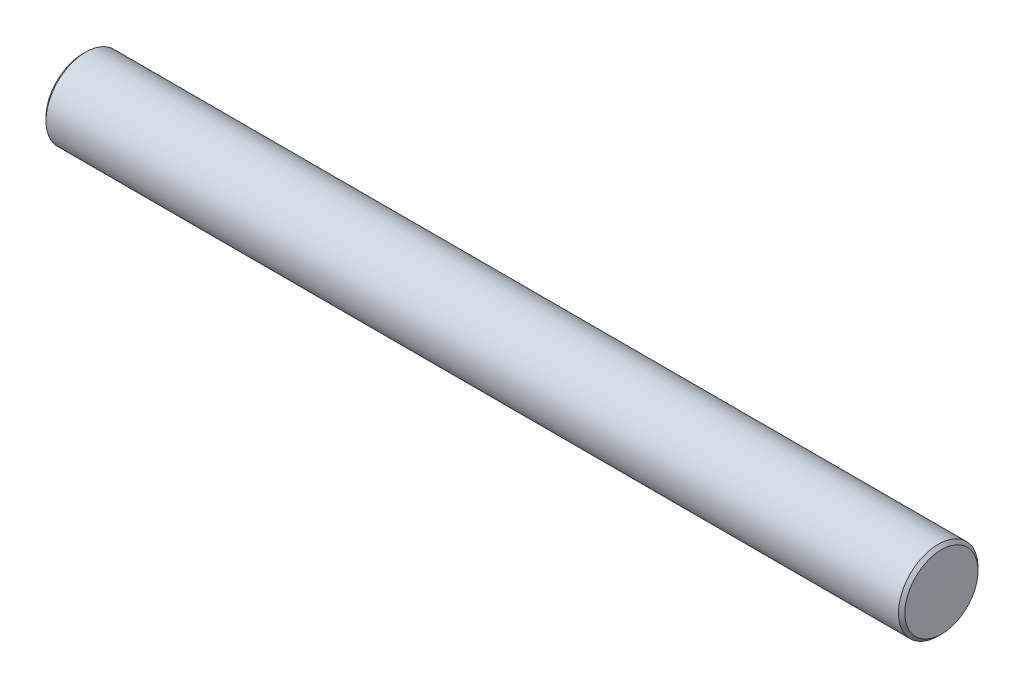
from build123d import *

# Parameters (mm, degrees)
SHAFT_HALF_PROFILE_W   = 540
SHAFT_HALF_PROFILE_H   = 25
END_CHAMFERS_2X45_SIZE = 2


with BuildPart() as part:
    # Shaft Half Profile → Shaft Ø50x540 (revolve)
    with BuildSketch(Plane.XY, mode=Mode.PRIVATE) as shaft_50x540_sk:
        with Locations((0, 12.5)):
            Rectangle(SHAFT_HALF_PROFILE_W, SHAFT_HALF_PROFILE_H)
    revolve(shaft_50x540_sk.sketch.rotate(Axis((-270, 0, 0), (1, 0, 0)), 180), axis=Axis((-270, 0, 0), (1, 0, 0)))

    # End Chamfers 2x45°
    end_chamfers_2x45_edges = [part.edges().sort_by_distance(p)[0] for p in [
        (-270, 25, 0),
        (270, 25, 0),
    ]]
    chamfer(end_chamfers_2x45_edges, length=END_CHAMFERS_2X45_SIZE)


solid = part.part
